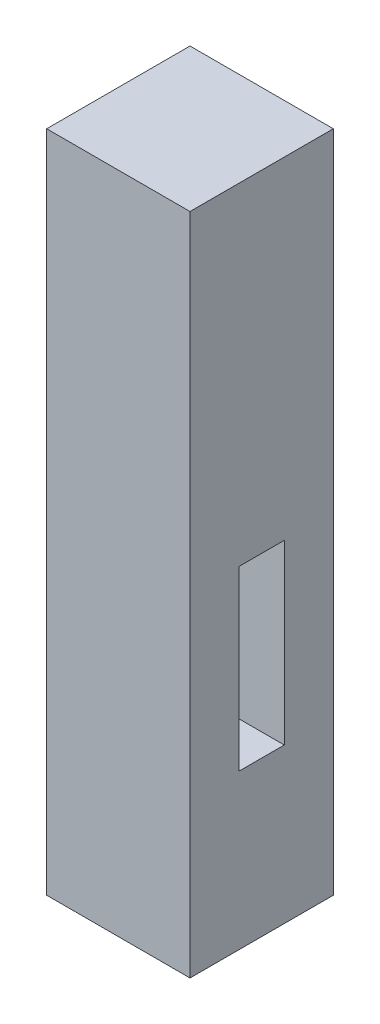
from build123d import *

# Parameters (mm, degrees)
ROD_SECTION_SKETCH_38X38_W = 38
ROD_SECTION_SKETCH_38X38_H = 38
SQUARE_ROD_38X38X176_DEPTH = 176
SLOT_PROFILE_SKETCH_W      = 12
SLOT_PROFILE_SKETCH_H      = 47
THROUGH_SLOT_47X12_DEPTH   = 176


with BuildPart() as part:
    # Rod Section Sketch 38x38 → Square Rod 38x38x176 (new body)
    with BuildSketch(Plane(origin=(0, 0, 0), x_dir=(1, 0, 0), z_dir=(0, 1, 0))):
        Rectangle(ROD_SECTION_SKETCH_38X38_W, ROD_SECTION_SKETCH_38X38_H)
    extrude(amount=SQUARE_ROD_38X38X176_DEPTH)

    # Slot Profile Sketch → Through Slot 47x12 (cut)
    with BuildSketch(Plane(origin=(19, 0, 0), x_dir=(0, 0, -1), z_dir=(1, 0, 0))):
        with Locations((0, 64.5)):
            Rectangle(SLOT_PROFILE_SKETCH_W, SLOT_PROFILE_SKETCH_H)
    extrude(amount=-THROUGH_SLOT_47X12_DEPTH, mode=Mode.SUBTRACT)


solid = part.part
